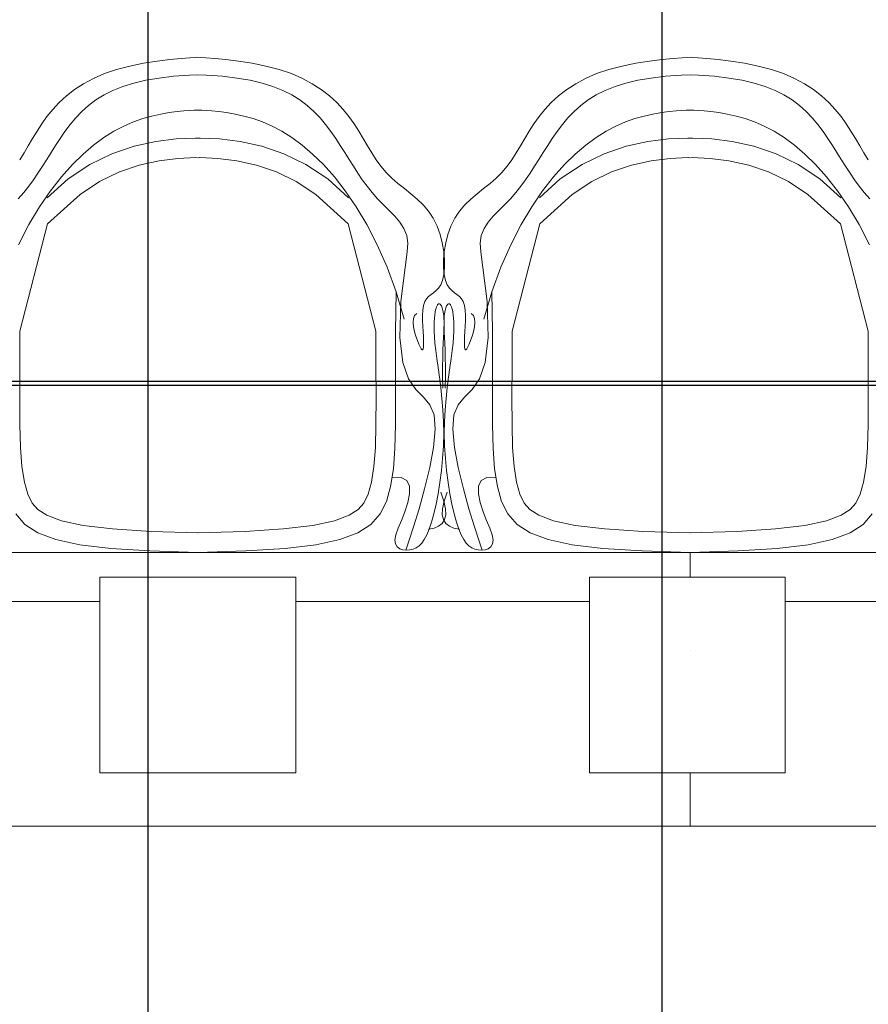
# Model space of a CAD drawing. Units: inches. Extents: x 1454 to 2136, y 626 to 1213.
# Tile 11 of 23: x 1620 to 1654, y 1101 to 1141. Entities that reach past the tile are written whole.
import ezdxf

# ---------------------------------------------------------------- set-up
doc = ezdxf.new("R2010")
doc.units = ezdxf.units.IN
doc.header["$MEASUREMENT"] = 0
for name, color, linetype, lineweight in [('A-ANNO-DIMS', 2, 'Continuous', 18), ('A-FURN-PATT', 252, 'Continuous', 13), ('conference', 41, 'Continuous', 18)]:
    doc.layers.add(name, color=color, linetype=linetype, lineweight=lineweight)
doc.styles.get("Standard").update_dxf_attribs({"font": 'arial.ttf'})
doc.dimstyles.get("Standard").update_dxf_attribs({"dimtxt": 4, "dimasz": 0.18, "dimexe": 0.18, "dimexo": 0.0625, "dimgap": 0.09, "dimtad": 0, "dimtih": 1, "dimtoh": 1, "dimdec": 0, "dimrnd": 6, "dimzin": 0, "dimdsep": 46, "dimlunit": 3, "dimtxsty": 'Standard', "dimcen": 0.09, "dimadec": 0, "dimazin": 0, "dimtfac": 1, "dimtdec": 0, "dimtofl": 0, "dimtmove": 0, "dimatfit": 3, "dimfxl": 1, "dimtolj": 1, "dimtzin": 0, "dimarcsym": 0})

# ---------------------------------------------------------------- blocks, each defined once
blk = doc.blocks.new('ОГ52_на12персон_стол2800х900')
for p, q in [((-520.6, 783.7), (-511.5, 784.5)), ((-511.5, 784.5), (-505.6, 784.9)), ((-505.6, 784.9), (-503.4, 785)), ((-501.2, 784.9), (-503.4, 785)), ((-495.2, 784.5), (-501.2, 784.9)), ((-486.2, 783.7), (-495.2, 784.5)), ((-17.8, 783.7), (-8.8, 784.5)), ((-8.8, 784.5), (-2.8, 784.9)), ((-2.8, 784.9), (-0.6, 785)), ((1.6, 784.9), (-0.6, 785)), ((7.5, 784.5), (1.6, 784.9)), ((16.6, 783.7), (7.5, 784.5)), ((-586.4, 772.5), (-572.8, 776)), ((-572.8, 776), (-558.8, 778.8)), ((-558.8, 778.8), (-544.9, 780.9)), ((-544.9, 780.9), (-531.9, 782.6)), ((-531.9, 782.6), (-520.6, 783.7)), ((-474.8, 782.6), (-486.2, 783.7)), ((-461.8, 780.9), (-474.8, 782.6)), ((-448, 778.8), (-461.8, 780.9)), ((-433.9, 776), (-448, 778.8)), ((-420.4, 772.5), (-433.9, 776)), ((-83.6, 772.5), (-70.1, 776)), ((-70.1, 776), (-56, 778.8)), ((-56, 778.8), (-42.2, 780.9)), ((-42.2, 780.9), (-29.2, 782.6)), ((-29.2, 782.6), (-17.8, 783.7)), ((27.9, 782.6), (16.6, 783.7)), ((40.9, 780.9), (27.9, 782.6)), ((54.8, 778.8), (40.9, 780.9)), ((68.8, 776), (54.8, 778.8)), ((82.4, 772.5), (68.8, 776)), ((-610.1, 763.4), (-598.8, 768.3)), ((-598.8, 768.3), (-586.4, 772.5)), ((-543.1, 763.8), (-528.3, 765.6)), ((-528.3, 765.6), (-512, 766.8)), ((-512, 766.8), (-503.4, 767.1)), ((-494.8, 766.8), (-503.4, 767.1)), ((-478.4, 765.6), (-494.8, 766.8)), ((-463.6, 763.8), (-478.4, 765.6)), ((-407.9, 768.3), (-420.4, 772.5)), ((-396.6, 763.4), (-407.9, 768.3)), ((-107.4, 763.4), (-96.1, 768.3)), ((-96.1, 768.3), (-83.6, 772.5)), ((-40.4, 763.8), (-25.6, 765.6)), ((-25.6, 765.6), (-9.3, 766.8)), ((-9.3, 766.8), (-0.6, 767.1)), ((8, 766.8), (-0.6, 767.1)), ((24.3, 765.6), (8, 766.8)), ((39.1, 763.8), (24.3, 765.6)), ((94.8, 768.3), (82.4, 772.5)), ((106.1, 763.4), (94.8, 768.3)), ((-629.5, 752), (-620.3, 758)), ((-620.3, 758), (-610.1, 763.4)), ((-590.1, 751.2), (-580, 755.2)), ((-580, 755.2), (-568.9, 758.7)), ((-568.9, 758.7), (-556.7, 761.5)), ((-556.7, 761.5), (-543.1, 763.8)), ((-450.1, 761.5), (-463.6, 763.8)), ((-437.8, 758.7), (-450.1, 761.5)), ((-426.7, 755.2), (-437.8, 758.7)), ((-416.6, 751.2), (-426.7, 755.2)), ((-386.5, 758), (-396.6, 763.4)), ((-377.3, 752), (-386.5, 758)), ((-126.7, 752), (-117.5, 758)), ((-117.5, 758), (-107.4, 763.4)), ((-87.4, 751.2), (-77.3, 755.2)), ((-77.3, 755.2), (-66.2, 758.7)), ((-66.2, 758.7), (-53.9, 761.5)), ((-53.9, 761.5), (-40.4, 763.8)), ((52.7, 761.5), (39.1, 763.8)), ((64.9, 758.7), (52.7, 761.5)), ((76, 755.2), (64.9, 758.7)), ((86.1, 751.2), (76, 755.2)), ((116.3, 758), (106.1, 763.4)), ((125.5, 752), (116.3, 758)), ((-645.1, 738.8), (-637.7, 745.6)), ((-637.7, 745.6), (-629.5, 752)), ((-607.5, 741.4), (-599.2, 746.6)), ((-599.2, 746.6), (-590.1, 751.2)), ((-407.5, 746.6), (-416.6, 751.2)), ((-399.2, 741.4), (-407.5, 746.6)), ((-369, 745.6), (-377.3, 752)), ((-361.6, 738.8), (-369, 745.6)), ((-142.4, 738.8), (-135, 745.6)), ((-135, 745.6), (-126.7, 752)), ((-104.8, 741.4), (-96.5, 746.6)), ((-96.5, 746.6), (-87.4, 751.2)), ((95.2, 746.6), (86.1, 751.2)), ((103.5, 741.4), (95.2, 746.6)), ((133.7, 745.6), (125.5, 752)), ((141.1, 738.8), (133.7, 745.6)), ((-651.7, 731.7), (-645.1, 738.8)), ((-621.9, 729.6), (-615, 735.7)), ((-615, 735.7), (-607.5, 741.4)), ((-391.7, 735.7), (-399.2, 741.4)), ((-384.9, 729.6), (-391.7, 735.7)), ((-355, 731.7), (-361.6, 738.8)), ((-149, 731.7), (-142.4, 738.8)), ((-119.1, 729.6), (-112.3, 735.7)), ((-112.3, 735.7), (-104.8, 741.4)), ((111, 735.7), (103.5, 741.4)), ((117.9, 729.6), (111, 735.7)), ((147.7, 731.7), (141.1, 738.8)), ((-662.9, 716.9), (-657.6, 724.4)), ((-657.6, 724.4), (-651.7, 731.7)), ((-628.1, 723.1), (-621.9, 729.6)), ((-559.7, 722.3), (-550.4, 724.9)), ((-550.4, 724.9), (-541.3, 727)), ((-541.3, 727), (-532.7, 728.5)), ((-532.7, 728.5), (-524.7, 729.6)), ((-524.7, 729.6), (-517.7, 730.4)), ((-517.7, 730.4), (-511.8, 730.8)), ((-511.8, 730.8), (-507.3, 731)), ((-507.3, 731), (-504.4, 731.1)), ((-504.4, 731.1), (-503.4, 731.1)), ((-502.3, 731.1), (-503.4, 731.1)), ((-499.4, 731), (-502.3, 731.1)), ((-494.9, 730.8), (-499.4, 731)), ((-489.1, 730.4), (-494.9, 730.8)), ((-482, 729.6), (-489.1, 730.4)), ((-474.1, 728.5), (-482, 729.6)), ((-465.4, 727), (-474.1, 728.5)), ((-456.3, 724.9), (-465.4, 727)), ((-447, 722.3), (-456.3, 724.9)), ((-378.6, 723.1), (-384.9, 729.6)), ((-349.1, 724.4), (-355, 731.7)), ((-343.8, 716.9), (-349.1, 724.4)), ((-160.2, 716.9), (-154.9, 724.4)), ((-154.9, 724.4), (-149, 731.7)), ((-125.4, 723.1), (-119.1, 729.6)), ((-57, 722.3), (-47.7, 724.9)), ((-47.7, 724.9), (-38.6, 727)), ((-38.6, 727), (-29.9, 728.5)), ((-29.9, 728.5), (-22, 729.6)), ((-22, 729.6), (-14.9, 730.4)), ((-14.9, 730.4), (-9.1, 730.8)), ((-9.1, 730.8), (-4.6, 731)), ((-4.6, 731), (-1.7, 731.1)), ((-1.7, 731.1), (-0.6, 731.1)), ((0.4, 731.1), (-0.6, 731.1)), ((3.3, 731), (0.4, 731.1)), ((7.8, 730.8), (3.3, 731)), ((13.7, 730.4), (7.8, 730.8)), ((20.7, 729.6), (13.7, 730.4)), ((28.7, 728.5), (20.7, 729.6)), ((37.3, 727), (28.7, 728.5)), ((46.4, 724.9), (37.3, 727)), ((55.7, 722.3), (46.4, 724.9)), ((124.1, 723.1), (117.9, 729.6)), ((153.6, 724.4), (147.7, 731.7)), ((158.9, 716.9), (153.6, 724.4)), ((-667.7, 709.4), (-662.9, 716.9)), ((-639.2, 709.3), (-633.9, 716.3)), ((-633.9, 716.3), (-628.1, 723.1)), ((-589.1, 709.4), (-579.1, 714.7)), ((-579.1, 714.7), (-569.3, 718.9)), ((-569.3, 718.9), (-559.7, 722.3)), ((-437.4, 718.9), (-447, 722.3)), ((-427.6, 714.7), (-437.4, 718.9)), ((-417.6, 709.4), (-427.6, 714.7)), ((-372.9, 716.3), (-378.6, 723.1)), ((-367.6, 709.3), (-372.9, 716.3)), ((-339, 709.4), (-343.8, 716.9)), ((-165, 709.4), (-160.2, 716.9)), ((-136.4, 709.3), (-131.1, 716.3)), ((-131.1, 716.3), (-125.4, 723.1)), ((-86.4, 709.4), (-76.4, 714.7)), ((-76.4, 714.7), (-66.6, 718.9)), ((-66.6, 718.9), (-57, 722.3)), ((65.3, 718.9), (55.7, 722.3)), ((75.1, 714.7), (65.3, 718.9)), ((85.1, 709.4), (75.1, 714.7)), ((129.8, 716.3), (124.1, 723.1)), ((135.2, 709.3), (129.8, 716.3)), ((163.7, 709.4), (158.9, 716.9)), ((-672.2, 701.9), (-667.7, 709.4)), ((-644.1, 702.2), (-639.2, 709.3)), ((-599.4, 703), (-589.1, 709.4)), ((-407.4, 703), (-417.6, 709.4)), ((-362.6, 702.2), (-367.6, 709.3)), ((-334.5, 701.9), (-339, 709.4)), ((-169.5, 701.9), (-165, 709.4)), ((-141.4, 702.2), (-136.4, 709.3)), ((-96.6, 703), (-86.4, 709.4)), ((95.4, 703), (85.1, 709.4)), ((140.1, 702.2), (135.2, 709.3)), ((168.2, 701.9), (163.7, 709.4)), ((-680.9, 687.3), (-676.6, 694.5)), ((-676.6, 694.5), (-672.2, 701.9)), ((-653.4, 687.9), (-648.8, 695)), ((-648.8, 695), (-644.1, 702.2)), ((-620.6, 686.1), (-609.9, 695.3)), ((-609.9, 695.3), (-599.4, 703)), ((-591.2, 686.5), (-568.6, 694.2)), ((-568.6, 694.2), (-546.5, 699)), ((-546.5, 699), (-525.4, 701.6)), ((-525.4, 701.6), (-505.7, 702.5)), ((-505.7, 702.5), (-503.4, 702.4)), ((-501, 702.5), (-503.4, 702.4)), ((-481.3, 701.6), (-501, 702.5)), ((-460.2, 699), (-481.3, 701.6)), ((-438.1, 694.2), (-460.2, 699)), ((-415.6, 686.5), (-438.1, 694.2)), ((-396.9, 695.3), (-407.4, 703)), ((-386.2, 686.1), (-396.9, 695.3)), ((-357.9, 695), (-362.6, 702.2)), ((-353.4, 687.9), (-357.9, 695)), ((-330.2, 694.5), (-334.5, 701.9)), ((-325.8, 687.3), (-330.2, 694.5)), ((-178.2, 687.3), (-173.9, 694.5)), ((-173.9, 694.5), (-169.5, 701.9)), ((-150.6, 687.9), (-146.1, 695)), ((-146.1, 695), (-141.4, 702.2)), ((-117.9, 686.1), (-107.1, 695.3)), ((-107.1, 695.3), (-96.6, 703)), ((-88.4, 686.5), (-65.9, 694.2)), ((-65.9, 694.2), (-43.8, 699)), ((-43.8, 699), (-22.7, 701.6)), ((-22.7, 701.6), (-3, 702.5)), ((-3, 702.5), (-0.6, 702.4)), ((1.7, 702.5), (-0.6, 702.4)), ((21.4, 701.6), (1.7, 702.5)), ((42.5, 699), (21.4, 701.6)), ((64.6, 694.2), (42.5, 699)), ((87.2, 686.5), (64.6, 694.2)), ((105.9, 695.3), (95.4, 703)), ((116.6, 686.1), (105.9, 695.3)), ((144.8, 695), (140.1, 702.2)), ((149.4, 687.9), (144.8, 695)), ((172.6, 694.5), (168.2, 701.9)), ((176.9, 687.3), (172.6, 694.5)), ((-685.4, 680.3), (-680.9, 687.3)), ((-657.8, 680.7), (-653.4, 687.9)), ((-631.5, 675.4), (-620.6, 686.1)), ((-613.8, 675.6), (-591.2, 686.5)), ((-393, 675.6), (-415.6, 686.5)), ((-375.2, 675.4), (-386.2, 686.1)), ((-348.9, 680.7), (-353.4, 687.9)), ((-321.3, 680.3), (-325.8, 687.3)), ((-182.7, 680.3), (-178.2, 687.3)), ((-155.1, 680.7), (-150.6, 687.9)), ((-128.8, 675.4), (-117.9, 686.1)), ((-111, 675.6), (-88.4, 686.5)), ((109.8, 675.6), (87.2, 686.5)), ((127.5, 675.4), (116.6, 686.1)), ((153.8, 680.7), (149.4, 687.9)), ((181.4, 680.3), (176.9, 687.3)), ((-666.7, 666.7), (-662.2, 673.7)), ((-662.2, 673.7), (-657.8, 680.7)), ((-642.7, 663), (-631.5, 675.4)), ((-636, 660.8), (-613.8, 675.6)), ((-583.6, 668), (-563.2, 674.9)), ((-563.2, 674.9), (-543.1, 679.3)), ((-543.1, 679.3), (-523.8, 681.7)), ((-523.8, 681.7), (-505.5, 682.5)), ((-505.5, 682.5), (-503.8, 682.4)), ((-501.3, 682.5), (-503, 682.4)), ((-483, 681.7), (-501.3, 682.5)), ((-463.6, 679.3), (-483, 681.7)), ((-443.5, 674.9), (-463.6, 679.3)), ((-423.2, 668), (-443.5, 674.9)), ((-370.7, 660.8), (-393, 675.6)), ((-364, 663), (-375.2, 675.4)), ((-344.5, 673.7), (-348.9, 680.7)), ((-340.1, 666.7), (-344.5, 673.7)), ((-316.5, 673.7), (-321.3, 680.3)), ((-311.2, 667.5), (-316.5, 673.7)), ((-192.8, 667.5), (-187.5, 673.7)), ((-187.5, 673.7), (-182.7, 680.3)), ((-163.9, 666.7), (-159.5, 673.7)), ((-159.5, 673.7), (-155.1, 680.7)), ((-140, 663), (-128.8, 675.4)), ((-133.3, 660.8), (-111, 675.6)), ((-80.8, 668), (-60.5, 674.9)), ((-60.5, 674.9), (-40.4, 679.3)), ((-40.4, 679.3), (-21, 681.7)), ((-21, 681.7), (-2.7, 682.5)), ((-2.7, 682.5), (-1, 682.4)), ((1.5, 682.5), (-0.2, 682.4)), ((19.7, 681.7), (1.5, 682.5)), ((39.1, 679.3), (19.7, 681.7)), ((59.2, 674.9), (39.1, 679.3)), ((79.6, 668), (59.2, 674.9)), ((132, 660.8), (109.8, 675.6)), ((138.7, 663), (127.5, 675.4)), ((158.2, 673.7), (153.8, 680.7)), ((162.7, 666.7), (158.2, 673.7)), ((-671.3, 659.9), (-666.7, 666.7)), ((-603.8, 658.2), (-583.6, 668)), ((-402.9, 658.2), (-423.2, 668)), ((-335.5, 659.9), (-340.1, 666.7)), ((-305.3, 661.7), (-311.2, 667.5)), ((-198.7, 661.7), (-192.8, 667.5)), ((-168.6, 659.9), (-163.9, 666.7)), ((-101.1, 658.2), (-80.8, 668)), ((99.8, 658.2), (79.6, 668)), ((167.3, 659.9), (162.7, 666.7)), ((-676.1, 653.3), (-671.3, 659.9)), ((-657.3, 641.6), (-636, 660.8)), ((-654, 648.7), (-642.7, 663)), ((-623.7, 644.9), (-603.8, 658.2)), ((-383, 644.9), (-402.9, 658.2)), ((-349.4, 641.6), (-370.7, 660.8)), ((-352.8, 648.7), (-364, 663)), ((-330.6, 653.3), (-335.5, 659.9)), ((-299, 656.2), (-305.3, 661.7)), ((-292.5, 650.9), (-299, 656.2)), ((-211.5, 650.9), (-205, 656.2)), ((-205, 656.2), (-198.7, 661.7)), ((-173.4, 653.3), (-168.6, 659.9)), ((-154.6, 641.6), (-133.3, 660.8)), ((-151.3, 648.7), (-140, 663)), ((-121, 644.9), (-101.1, 658.2)), ((119.7, 644.9), (99.8, 658.2)), ((153.3, 641.6), (132, 660.8)), ((150, 648.7), (138.7, 663)), ((172.1, 653.3), (167.3, 659.9)), ((-686.8, 640.6), (-681.3, 646.8)), ((-681.3, 646.8), (-676.1, 653.3)), ((-665.2, 632.4), (-654, 648.7)), ((-657, 615), (-623.7, 644.9)), ((-349.8, 615), (-383, 644.9)), ((-341.6, 632.4), (-352.8, 648.7)), ((-325.5, 646.8), (-330.6, 653.3)), ((-320, 640.6), (-325.5, 646.8)), ((-285.9, 645.6), (-292.5, 650.9)), ((-279.5, 640.1), (-285.9, 645.6)), ((-224.5, 640.1), (-218.1, 645.6)), ((-218.1, 645.6), (-211.5, 650.9)), ((-184, 640.6), (-178.5, 646.8)), ((-178.5, 646.8), (-173.4, 653.3)), ((-162.4, 632.4), (-151.3, 648.7)), ((-154.2, 615), (-121, 644.9)), ((153, 615), (119.7, 644.9)), ((161.2, 632.4), (150, 648.7)), ((177.3, 646.8), (172.1, 653.3)), ((182.8, 640.6), (177.3, 646.8)), ((-314.1, 634.6), (-320, 640.6)), ((-308, 628.7), (-314.1, 634.6)), ((-273.4, 634.2), (-279.5, 640.1)), ((-267.8, 627.7), (-273.4, 634.2)), ((-236.2, 627.7), (-230.6, 634.2)), ((-230.6, 634.2), (-224.5, 640.1)), ((-196, 628.7), (-190, 634.6)), ((-190, 634.6), (-184, 640.6)), ((-676.1, 614.1), (-665.2, 632.4)), ((-330.7, 614.1), (-341.6, 632.4)), ((-302.3, 622.8), (-308, 628.7)), ((-263, 620.6), (-267.8, 627.7)), ((-241, 620.6), (-236.2, 627.7)), ((-201.7, 622.8), (-196, 628.7)), ((-173.3, 614.1), (-162.4, 632.4)), ((172.1, 614.1), (161.2, 632.4)), ((-686.6, 593.6), (-676.1, 614.1)), ((-657, 615), (-685.3, 505.2)), ((-349.8, 615), (-321.5, 505.2)), ((-320.1, 593.6), (-330.7, 614.1)), ((-297.1, 616.6), (-302.3, 622.8)), ((-292.9, 610.1), (-297.1, 616.6)), ((-259.1, 612.7), (-263, 620.6)), ((-244.9, 612.7), (-241, 620.6)), ((-211.1, 610.1), (-206.9, 616.6)), ((-206.9, 616.6), (-201.7, 622.8)), ((-183.9, 593.6), (-173.3, 614.1)), ((-154.2, 615), (-182.5, 505.2)), ((153, 615), (181.3, 505.2)), ((182.6, 593.6), (172.1, 614.1)), ((-290, 603), (-292.9, 610.1)), ((-256, 604.2), (-259.1, 612.7)), ((-253.8, 595.4), (-256, 604.2)), ((-250.2, 595.4), (-248, 604.2)), ((-248, 604.2), (-244.9, 612.7)), ((-214, 603), (-211.1, 610.1)), ((-310.2, 570.7), (-320.1, 593.6)), ((-288.8, 595.2), (-290, 603)), ((-289.6, 586.5), (-288.8, 595.2)), ((-252.3, 586.6), (-253.8, 595.4)), ((-251.7, 586.6), (-250.2, 595.4)), ((-215.2, 595.2), (-214, 603)), ((-214.4, 586.5), (-215.2, 595.2)), ((-193.8, 570.7), (-183.9, 593.6)), ((-289.6, 586.5), (-296, 535.5)), ((-252.4, 578.1), (-251.7, 586.6)), ((-251.6, 578.1), (-252.3, 586.6)), ((-214.4, 586.5), (-208, 535.5)), ((-252.4, 570.2), (-252.4, 578.1)), ((-251.6, 570.2), (-251.6, 578.1)), ((-301, 545.4), (-310.2, 570.7)), ((-253.5, 557.2), (-252.3, 563.1)), ((-251.7, 563.1), (-252.4, 570.2)), ((-252.3, 563.1), (-251.6, 570.2)), ((-250.5, 557.2), (-251.7, 563.1)), ((-203, 545.4), (-193.8, 570.7)), ((-255.3, 552.7), (-253.5, 557.2)), ((-248.7, 552.7), (-250.5, 557.2)), ((-301, 545.4), (-301.5, 505.1)), ((-292.7, 517.6), (-301, 545.4)), ((-265.2, 542.8), (-262.6, 544.6)), ((-262.6, 544.6), (-260, 546.7)), ((-260, 546.7), (-257.5, 549.3)), ((-257.5, 549.3), (-255.3, 552.7)), ((-246.5, 549.3), (-248.7, 552.7)), ((-244, 546.7), (-246.5, 549.3)), ((-241.4, 544.6), (-244, 546.7)), ((-238.8, 542.8), (-241.4, 544.6)), ((-211.3, 517.6), (-203, 545.4)), ((-203, 545.4), (-202.5, 505.1)), ((-296, 535.5), (-297, 498.8)), ((-272.8, 531.5), (-271.6, 535.5)), ((-271.6, 535.5), (-269.8, 538.5)), ((-269.8, 538.5), (-267.7, 540.8)), ((-267.7, 540.8), (-265.2, 542.8)), ((-258.6, 532.3), (-258.1, 532.9)), ((-258.1, 532.9), (-257.6, 533.2)), ((-257.6, 533.2), (-257, 533.3)), ((-257, 533.3), (-256.5, 533.2)), ((-256.5, 533.2), (-256, 533)), ((-256, 533), (-255.6, 532.5)), ((-248, 533), (-248.4, 532.5)), ((-247.5, 533.2), (-248, 533)), ((-247, 533.3), (-247.5, 533.2)), ((-246.4, 533.2), (-247, 533.3)), ((-245.9, 532.9), (-246.4, 533.2)), ((-245.4, 532.3), (-245.9, 532.9)), ((-236.3, 540.8), (-238.8, 542.8)), ((-234.2, 538.5), (-236.3, 540.8)), ((-232.4, 535.5), (-234.2, 538.5)), ((-231.2, 531.5), (-232.4, 535.5)), ((-208, 535.5), (-207, 498.8)), ((-279.9, 523.4), (-282.1, 521.4)), ((-273.8, 521.5), (-273.5, 526.8)), ((-273.5, 526.8), (-272.8, 531.5)), ((-261.4, 521.9), (-261, 524.7)), ((-261, 524.7), (-260.6, 527)), ((-260.6, 527), (-260.1, 528.8)), ((-260.1, 528.8), (-259.6, 530.3)), ((-259.6, 530.3), (-259.1, 531.5)), ((-259.1, 531.5), (-258.6, 532.3)), ((-255.6, 532.5), (-255.1, 531.9)), ((-255.1, 531.9), (-254.7, 531.1)), ((-254.7, 531.1), (-254.2, 530.2)), ((-254.2, 530.2), (-253.8, 529.1)), ((-253.8, 529.1), (-253.5, 527.9)), ((-253.5, 527.9), (-253.1, 526.5)), ((-253.1, 526.5), (-252.8, 524.9)), ((-252.8, 524.9), (-252.5, 523.1)), ((-252.5, 523.1), (-252.3, 521)), ((-251.5, 523.1), (-251.7, 521)), ((-251.2, 524.9), (-251.5, 523.1)), ((-250.9, 526.5), (-251.2, 524.9)), ((-250.6, 527.9), (-250.9, 526.5)), ((-250.2, 529.1), (-250.6, 527.9)), ((-249.8, 530.2), (-250.2, 529.1)), ((-249.3, 531.1), (-249.8, 530.2)), ((-248.9, 531.9), (-249.3, 531.1)), ((-248.4, 532.5), (-248.9, 531.9)), ((-244.9, 531.5), (-245.4, 532.3)), ((-244.4, 530.3), (-244.9, 531.5)), ((-243.9, 528.8), (-244.4, 530.3)), ((-243.4, 527), (-243.9, 528.8)), ((-243, 524.7), (-243.4, 527)), ((-242.6, 521.9), (-243, 524.7)), ((-230.5, 526.8), (-231.2, 531.5)), ((-230.2, 521.5), (-230.5, 526.8)), ((-224.1, 523.4), (-221.9, 521.4)), ((-283.2, 518.2), (-283.5, 514.2)), ((-283.5, 514.2), (-283, 509.6)), ((-282.1, 521.4), (-283.2, 518.2)), ((-273.8, 516), (-273.8, 521.5)), ((-273.6, 510.3), (-273.8, 516)), ((-262, 510.5), (-261.9, 514.9)), ((-261.9, 514.9), (-261.7, 518.7)), ((-261.7, 518.7), (-261.4, 521.9)), ((-252.3, 521), (-252.1, 518.5)), ((-252.1, 518.5), (-252, 515.7)), ((-251.9, 518.5), (-252, 515.7)), ((-252, 515.7), (-252, 512.3)), ((-252, 515.7), (-252, 512.3)), ((-251.7, 521), (-251.9, 518.5)), ((-242.3, 518.7), (-242.6, 521.9)), ((-242.1, 514.9), (-242.3, 518.7)), ((-242, 510.5), (-242.1, 514.9)), ((-230.4, 510.3), (-230.2, 516)), ((-230.2, 516), (-230.2, 521.5)), ((-221.9, 521.4), (-220.8, 518.2)), ((-220.5, 514.2), (-221, 509.6)), ((-220.8, 518.2), (-220.5, 514.2)), ((-685.3, 505.2), (-685.3, 469.2)), ((-321.5, 505.2), (-321.5, 469.2)), ((-301.5, 505.1), (-301.5, 469.2)), ((-283, 509.6), (-282, 504.8)), ((-282, 504.8), (-280.7, 500.1)), ((-273.4, 504.9), (-273.6, 510.3)), ((-273.1, 499.8), (-273.4, 504.9)), ((-262, 505.4), (-262, 510.5)), ((-261.7, 499.6), (-262, 505.4)), ((-252.3, 504), (-252.5, 498.9)), ((-252.1, 508.5), (-252.3, 504)), ((-252, 512.3), (-252.1, 508.5)), ((-252, 512.3), (-251.9, 508.5)), ((-251.9, 508.5), (-251.7, 504)), ((-251.7, 504), (-251.5, 498.9)), ((-242.3, 499.6), (-242, 505.4)), ((-242, 505.4), (-242, 510.5)), ((-230.9, 499.8), (-230.6, 504.9)), ((-230.6, 504.9), (-230.4, 510.3)), ((-222, 504.8), (-223.3, 500.1)), ((-221, 509.6), (-222, 504.8)), ((-202.5, 505.1), (-202.5, 469.2)), ((-182.5, 505.2), (-182.5, 469.2)), ((181.3, 505.2), (181.3, 469.2)), ((-297, 498.8), (-294, 473.4)), ((-280.7, 500.1), (-279.2, 495.7)), ((-279.2, 495.7), (-277.7, 492)), ((-272.9, 495.4), (-273.1, 499.8)), ((-272.8, 491.8), (-272.9, 495.4)), ((-261.2, 493.1), (-261.7, 499.6)), ((-260.4, 485.6), (-261.2, 493.1)), ((-252.8, 493), (-253.1, 486.1)), ((-252.5, 498.9), (-252.8, 493)), ((-251.5, 498.9), (-251.2, 493)), ((-251.2, 493), (-250.9, 486.1)), ((-243.6, 485.6), (-242.8, 493.1)), ((-242.8, 493.1), (-242.3, 499.6)), ((-231.2, 491.8), (-231.1, 495.4)), ((-231.1, 495.4), (-230.9, 499.8)), ((-224.8, 495.7), (-226.3, 492)), ((-223.3, 500.1), (-224.8, 495.7)), ((-207, 498.8), (-210.1, 473.4)), ((-277.7, 492), (-276.4, 489.2)), ((-276.4, 489.2), (-275.3, 487.3)), ((-275.3, 487.3), (-274.4, 486.4)), ((-274.4, 486.4), (-273.8, 486.4)), ((-273.8, 486.4), (-273.3, 487.3)), ((-273.3, 487.3), (-272.9, 489.1)), ((-272.9, 489.1), (-272.8, 491.8)), ((-259.3, 477.3), (-260.4, 485.6)), ((-253.1, 486.1), (-253.3, 478.2)), ((-250.9, 486.1), (-250.7, 478.2)), ((-244.7, 477.3), (-243.6, 485.6)), ((-231.1, 489.1), (-231.2, 491.8)), ((-230.7, 487.3), (-231.1, 489.1)), ((-230.3, 486.4), (-230.7, 487.3)), ((-229.6, 486.4), (-230.3, 486.4)), ((-228.7, 487.3), (-229.6, 486.4)), ((-227.6, 489.2), (-228.7, 487.3)), ((-226.3, 492), (-227.6, 489.2)), ((-294, 473.4), (-288.1, 456.6)), ((-258, 468.2), (-259.3, 477.3)), ((-253.3, 478.2), (-253.4, 469.2)), ((-250.7, 478.2), (-250.6, 469.2)), ((-246, 468.2), (-244.7, 477.3)), ((-210.1, 473.4), (-215.9, 456.6)), ((-685.3, 469.2), (-685.4, 437.6)), ((-321.5, 469.2), (-321.4, 437.6)), ((-301.5, 469.2), (-301.4, 437.5)), ((-256.7, 458.3), (-258, 468.2)), ((-253.4, 469.2), (-253.5, 458.8)), ((-250.6, 469.2), (-250.5, 458.8)), ((-247.3, 458.3), (-246, 468.2)), ((-202.5, 469.2), (-202.6, 437.5)), ((-182.5, 469.2), (-182.6, 437.6)), ((181.3, 469.2), (181.4, 437.6)), ((-288.1, 456.6), (-280.7, 445.7)), ((-255.4, 447.8), (-256.7, 458.3)), ((-253.5, 458.8), (-253.3, 447.1)), ((-250.5, 458.8), (-250.7, 447.1)), ((-248.7, 447.8), (-247.3, 458.3)), ((-215.9, 456.6), (-223.3, 445.7)), ((-280.7, 445.7), (-273.1, 437.8)), ((-254.1, 436.7), (-255.4, 447.8)), ((-249.9, 436.7), (-248.7, 447.8)), ((-223.3, 445.7), (-230.9, 437.8)), ((-685.4, 437.6), (-685.3, 410.1)), ((-321.4, 437.6), (-321.5, 410.1)), ((-301.4, 437.5), (-301.5, 409.8)), ((-273.1, 437.8), (-266.5, 430.2)), ((-253.1, 425.1), (-254.1, 436.7)), ((-250.9, 425.1), (-249.9, 436.7)), ((-230.9, 437.8), (-237.5, 430.2)), ((-202.6, 437.5), (-202.5, 409.8)), ((-182.6, 437.6), (-182.5, 410.1)), ((181.4, 437.6), (181.2, 410.1)), ((-266.5, 430.2), (-262.2, 420)), ((-252.5, 413.1), (-253.1, 425.1)), ((-251.5, 413.1), (-250.9, 425.1)), ((-237.5, 430.2), (-241.8, 420)), ((-262.2, 420), (-261.1, 405.3)), ((-252.3, 400.7), (-252.5, 413.1)), ((-251.7, 400.7), (-251.5, 413.1)), ((-241.8, 420), (-242.9, 405.3)), ((-685.3, 410.1), (-684.6, 386.6)), ((-321.5, 410.1), (-322.1, 386.6)), ((-301.5, 409.8), (-302.2, 385.6)), ((-261.1, 405.3), (-262.8, 386.7)), ((-242.9, 405.3), (-241.2, 386.7)), ((-202.5, 409.8), (-201.8, 385.6)), ((-182.5, 410.1), (-181.9, 386.6)), ((181.2, 410.1), (180.6, 386.6)), ((-252.6, 388.2), (-252.3, 400.7)), ((-251.4, 388.2), (-251.7, 400.7)), ((-684.6, 386.6), (-683.1, 367)), ((-322.1, 386.6), (-323.6, 367)), ((-302.2, 385.6), (-303.7, 364.7)), ((-262.8, 386.7), (-266.6, 366)), ((-253.4, 375.5), (-252.6, 388.2)), ((-250.6, 375.5), (-251.4, 388.2)), ((-241.2, 386.7), (-237.4, 366)), ((-201.8, 385.6), (-200.3, 364.7)), ((-181.9, 386.6), (-180.4, 367)), ((180.6, 386.6), (179.1, 367)), ((-254.6, 363), (-253.4, 375.5)), ((-249.4, 363), (-250.6, 375.5)), ((-683.1, 367), (-680.6, 351.1)), ((-323.6, 367), (-326.1, 351.1)), ((-303.7, 364.7), (-306.5, 346.8)), ((-266.6, 366), (-271.8, 344.5)), ((-256.2, 350.9), (-254.6, 363)), ((-247.8, 350.9), (-249.4, 363)), ((-237.4, 366), (-232.2, 344.5)), ((-200.3, 364.7), (-197.5, 346.8)), ((-180.4, 367), (-177.9, 351.1)), ((179.1, 367), (176.6, 351.1)), ((-295.6, 356.1), (-305.1, 355.7)), ((-289.9, 353), (-295.6, 356.1)), ((-287.3, 347.1), (-289.9, 353)), ((-216.7, 347.1), (-214.1, 353)), ((-214.1, 353), (-208.4, 356.1)), ((-208.4, 356.1), (-198.9, 355.7)), ((-680.6, 351.1), (-677.1, 338.8)), ((-326.1, 351.1), (-329.6, 338.8)), ((-306.5, 346.8), (-310.9, 331.5)), ((-287.3, 339.3), (-287.3, 347.1)), ((-271.8, 344.5), (-277.5, 323.8)), ((-258, 339.4), (-256.2, 350.9)), ((-246, 339.4), (-247.8, 350.9)), ((-232.2, 344.5), (-226.5, 323.8)), ((-216.7, 339.3), (-216.7, 347.1)), ((-197.5, 346.8), (-193.1, 331.5)), ((-177.9, 351.1), (-174.4, 338.8)), ((176.6, 351.1), (173.1, 338.8)), ((-677.1, 338.8), (-672.7, 329.9)), ((-329.6, 338.8), (-334, 329.9)), ((-289.1, 330.3), (-287.3, 339.3)), ((-260.1, 328.7), (-258, 339.4)), ((-255.4, 341), (-252.1, 331.8)), ((-251.9, 331.8), (-253.6, 324.1)), ((-252.1, 331.8), (-250.4, 324.1)), ((-248.6, 341), (-251.9, 331.8)), ((-243.9, 328.7), (-246, 339.4)), ((-214.9, 330.3), (-216.7, 339.3)), ((-174.4, 338.8), (-170, 329.9)), ((173.1, 338.8), (168.7, 329.9)), ((-672.7, 329.9), (-666.9, 323.3)), ((-666.9, 323.3), (-657.8, 317.4)), ((-339.8, 323.3), (-349, 317.4)), ((-334, 329.9), (-339.8, 323.3)), ((-310.9, 331.5), (-317.3, 318.7)), ((-292, 321), (-289.1, 330.3)), ((-277.5, 323.8), (-283.1, 305.4)), ((-262.3, 318.9), (-260.1, 328.7)), ((-253.6, 324.1), (-253.8, 317.8)), ((-250.4, 324.1), (-250.2, 317.8)), ((-241.7, 318.9), (-243.9, 328.7)), ((-226.5, 323.8), (-220.9, 305.4)), ((-212, 321), (-214.9, 330.3)), ((-193.1, 331.5), (-186.7, 318.7)), ((-170, 329.9), (-164.2, 323.3)), ((-164.2, 323.3), (-155.1, 317.4)), ((162.9, 323.3), (153.8, 317.4)), ((168.7, 329.9), (162.9, 323.3)), ((-689.5, 318.7), (-680.2, 308)), ((-657.8, 317.4), (-642.8, 311.8)), ((-642.8, 311.8), (-620.7, 307)), ((-363.9, 311.8), (-386.1, 307)), ((-349, 317.4), (-363.9, 311.8)), ((-317.3, 318.7), (-326.6, 308)), ((-298.9, 304.2), (-295.5, 312)), ((-295.5, 312), (-292, 321)), ((-264.7, 310.4), (-262.3, 318.9)), ((-251.5, 312.9), (-254, 309)), ((-253.8, 317.8), (-252.5, 312.9)), ((-252.5, 312.9), (-250, 309)), ((-250.2, 317.8), (-251.5, 312.9)), ((-239.3, 310.4), (-241.7, 318.9)), ((-208.5, 312), (-212, 321)), ((-205.1, 304.2), (-208.5, 312)), ((-186.7, 318.7), (-177.4, 308)), ((-155.1, 317.4), (-140.1, 311.8)), ((-140.1, 311.8), (-117.9, 307)), ((138.8, 311.8), (116.7, 307)), ((153.8, 317.4), (138.8, 311.8)), ((185.5, 318.7), (176.2, 308)), ((-680.2, 308), (-666.8, 299.4)), ((-620.7, 307), (-590.5, 303.4)), ((-590.5, 303.4), (-551.5, 300.9)), ((-416.3, 303.4), (-455.2, 300.9)), ((-386.1, 307), (-416.3, 303.4)), ((-326.6, 308), (-339.9, 299.4)), ((-298.9, 304.2), (-301.3, 297.4)), ((-283.1, 305.4), (-287.8, 291)), ((-269.5, 297.3), (-267.1, 303.2)), ((-262.2, 304.3), (-267.7, 303.1)), ((-267.1, 303.2), (-264.7, 310.4)), ((-257.6, 306.2), (-262.2, 304.3)), ((-254, 309), (-257.6, 306.2)), ((-250, 309), (-246.4, 306.2)), ((-246.4, 306.2), (-241.8, 304.3)), ((-241.8, 304.3), (-236.3, 303.1)), ((-236.9, 303.2), (-239.3, 310.4)), ((-234.5, 297.3), (-236.9, 303.2)), ((-220.9, 305.4), (-216.2, 291)), ((-205.1, 304.2), (-202.7, 297.4)), ((-177.4, 308), (-164.1, 299.4)), ((-117.9, 307), (-87.8, 303.4)), ((-87.8, 303.4), (-48.8, 300.9)), ((86.5, 303.4), (47.5, 300.9)), ((116.7, 307), (86.5, 303.4)), ((176.2, 308), (162.8, 299.4)), ((-666.8, 299.4), (-648.5, 292.5)), ((-648.5, 292.5), (-624, 287.3)), ((-551.5, 300.9), (-502.7, 299.3)), ((-455.2, 300.9), (-504, 299.3)), ((-358.3, 292.5), (-382.8, 287.3)), ((-339.9, 299.4), (-358.3, 292.5)), ((-301.3, 297.4), (-302.1, 292.1)), ((-302.1, 292.1), (-301.5, 288.1)), ((-274.7, 288.8), (-272.1, 292.5)), ((-272.1, 292.5), (-269.5, 297.3)), ((-231.9, 292.5), (-234.5, 297.3)), ((-229.3, 288.8), (-231.9, 292.5)), ((-202.7, 297.4), (-201.9, 292.1)), ((-201.9, 292.1), (-202.5, 288.1)), ((-164.1, 299.4), (-145.7, 292.5)), ((-145.7, 292.5), (-121.2, 287.3)), ((-48.8, 300.9), (0, 299.3)), ((47.5, 300.9), (-1.3, 299.3)), ((144.5, 292.5), (120, 287.3)), ((162.8, 299.4), (144.5, 292.5)), ((-624, 287.3), (-592.3, 283.5)), ((-592.3, 283.5), (-552.5, 280.9)), ((-414.4, 283.5), (-454.3, 280.9)), ((-382.8, 287.3), (-414.4, 283.5)), ((-301.5, 288.1), (-299.7, 285.1)), ((-299.7, 285.1), (-297.1, 283.2)), ((-297.1, 283.2), (-293.9, 282.2)), ((-293.9, 282.2), (-290.4, 281.8)), ((-287.8, 291), (-290.9, 281.9)), ((-290.4, 281.8), (-286.9, 282.1)), ((-286.9, 282.1), (-283.6, 282.8)), ((-283.6, 282.8), (-280.4, 284.1)), ((-280.4, 284.1), (-277.5, 286.1)), ((-277.5, 286.1), (-274.7, 288.8)), ((-226.5, 286.1), (-229.3, 288.8)), ((-223.6, 284.1), (-226.5, 286.1)), ((-220.4, 282.8), (-223.6, 284.1)), ((-217.1, 282.1), (-220.4, 282.8)), ((-213.6, 281.8), (-217.1, 282.1)), ((-216.2, 291), (-213.1, 281.9)), ((-210.1, 282.2), (-213.6, 281.8)), ((-206.9, 283.2), (-210.1, 282.2)), ((-204.3, 285.1), (-206.9, 283.2)), ((-202.5, 288.1), (-204.3, 285.1)), ((-121.2, 287.3), (-89.6, 283.5)), ((-89.6, 283.5), (-49.7, 280.9)), ((88.3, 283.5), (48.5, 280.9)), ((120, 287.3), (88.3, 283.5)), ((-1300, 279.3), (1300, 279.3)), ((-552.5, 280.9), (-503.4, 279.3)), ((-454.3, 280.9), (-503.4, 279.3)), ((-49.7, 280.9), (-0.6, 279.3)), ((48.5, 280.9), (-0.6, 279.3)), ((-0.6, 279.3), (-0.6, 254.3)), ((-603.4, 254.3), (-603.4, 54.3)), ((-403.4, 254.3), (-603.4, 254.3)), ((-403.4, 54.3), (-403.4, 254.3)), ((-103.4, 254.3), (-103.4, 54.3)), ((96.6, 254.3), (-103.4, 254.3)), ((96.6, 54.3), (96.6, 254.3)), ((-603.4, 229.3), (-903.4, 229.3)), ((-103.4, 229.3), (-403.4, 229.3)), ((403.4, 229.3), (96.6, 229.3)), ((0, 179.3), (0, 179.3)), ((0, 179.3), (0, 179.3)), ((-603.4, 54.3), (-403.4, 54.3)), ((-103.4, 54.3), (96.6, 54.3)), ((-0.6, 54.3), (-0.6, 0)), ((1220.7, 0), (-1220.7, 0))]:
    blk.add_line(p, q)
blk = doc.blocks.new('*D23')
at = {"layer": 'A-ANNO-DIMS', "color": 0, "lineweight": -2, "transparency": 16777216}
for p, q in [((1571.674, 1139.532), (1571.674, 1162.157)), ((1721.725, 1139.532), (1721.725, 1162.157)), ((1571.854, 1161.977), (1615.675, 1161.977)), ((1721.545, 1161.977), (1677.724, 1161.977))]:
    blk.add_line(p, q, dxfattribs=at)
at = {"layer": 'A-ANNO-DIMS', "color": 0, "transparency": 16777216}
for points in [[(1571.854, 1162.007), (1571.854, 1161.947), (1571.674, 1161.977)], [(1721.545, 1162.007), (1721.545, 1161.947), (1721.725, 1161.977)]]:
    blk.add_solid(points, dxfattribs=at)
at = {"layer": 'Defpoints', "color": 0, "transparency": 16777216}
for p in [(1721.725, 1161.977), (1571.674, 1139.469), (1721.725, 1139.469)]:
    blk.add_point(p, dxfattribs=at)
at = {"layer": 'A-ANNO-DIMS', "color": 0, "transparency": 16777216, "insert": (1646.7, 1161.977), "char_height": 4, "attachment_point": 5}
blk.add_mtext('\\A1;CONFERENCE SET 150', dxfattribs=at)
blk = doc.blocks.new('*D33')
at = {"layer": 'A-ANNO-DIMS', "color": 0, "lineweight": -2, "transparency": 16777216}
for p, q in [((2032.494, 1126.282), (1462.374, 1126.282)), ((1462.554, 1126.102), (1462.554, 1056.381)), ((1462.554, 982.462), (1462.554, 1052.184)), ((2032.494, 982.282), (1462.374, 982.282))]:
    blk.add_line(p, q, dxfattribs=at)
at = {"layer": 'A-ANNO-DIMS', "color": 0, "transparency": 16777216}
for points in [[(1462.524, 1126.102), (1462.584, 1126.102), (1462.554, 1126.282)], [(1462.524, 982.462), (1462.584, 982.462), (1462.554, 982.282)]]:
    blk.add_solid(points, dxfattribs=at)
at = {"layer": 'Defpoints', "color": 0, "transparency": 16777216}
for p in [(1462.554, 1126.282), (2032.556, 1126.282), (2032.556, 982.282)]:
    blk.add_point(p, dxfattribs=at)
at = {"layer": 'A-ANNO-DIMS', "color": 0, "transparency": 16777216, "insert": (1462.554, 1054.282), "char_height": 4, "attachment_point": 5}
blk.add_mtext('\\A1;144', dxfattribs=at)
blk = doc.blocks.new('*D40')
at = {"layer": 'A-ANNO-DIMS', "color": 0, "lineweight": -2, "transparency": 16777216}
for p, q in [((1501.556, 877.345), (1501.556, 1210.464)), ((1501.736, 1210.284), (1569.244, 1210.284)), ((1645.376, 1210.284), (1577.869, 1210.284)), ((1645.556, 877.345), (1645.556, 1210.464))]:
    blk.add_line(p, q, dxfattribs=at)
at = {"layer": 'A-ANNO-DIMS', "color": 0, "transparency": 16777216}
for points in [[(1501.736, 1210.314), (1501.736, 1210.254), (1501.556, 1210.284)], [(1645.376, 1210.314), (1645.376, 1210.254), (1645.556, 1210.284)]]:
    blk.add_solid(points, dxfattribs=at)
at = {"layer": 'Defpoints', "color": 0, "transparency": 16777216}
for p in [(1645.556, 1210.284), (1501.556, 877.282), (1645.556, 877.282)]:
    blk.add_point(p, dxfattribs=at)
at = {"layer": 'A-ANNO-DIMS', "color": 0, "transparency": 16777216, "insert": (1573.556, 1210.284), "char_height": 4, "attachment_point": 5}
blk.add_mtext('\\A1;144', dxfattribs=at)
blk = doc.blocks.new('*D54')
at = {"layer": 'A-ANNO-DIMS', "color": 0, "lineweight": -2, "transparency": 16777216}
for p, q in [((1879.494, 1126.282), (1462.374, 1126.282)), ((1462.554, 1126.102), (1462.554, 1078.915)), ((1462.554, 1027.462), (1462.554, 1074.65)), ((1879.494, 1027.282), (1462.374, 1027.282))]:
    blk.add_line(p, q, dxfattribs=at)
at = {"layer": 'A-ANNO-DIMS', "color": 0, "transparency": 16777216}
for points in [[(1462.524, 1126.102), (1462.584, 1126.102), (1462.554, 1126.282)], [(1462.524, 1027.462), (1462.584, 1027.462), (1462.554, 1027.282)]]:
    blk.add_solid(points, dxfattribs=at)
at = {"layer": 'Defpoints', "color": 0, "transparency": 16777216}
for p in [(1879.556, 1126.282), (1462.554, 1027.282), (1879.556, 1027.282)]:
    blk.add_point(p, dxfattribs=at)
at = {"layer": 'A-ANNO-DIMS', "color": 0, "transparency": 16777216, "insert": (1462.554, 1076.782), "char_height": 4, "attachment_point": 5}
blk.add_mtext('\\A1;99', dxfattribs=at)
blk = doc.blocks.new('*D67')
at = {"layer": 'A-ANNO-DIMS', "color": 0, "lineweight": -2, "transparency": 16777216}
for p, q in [((1606.484, 1018.345), (1606.484, 1210.464)), ((1606.664, 1210.284), (1610.595, 1210.284)), ((1624.703, 1210.284), (1620.773, 1210.284)), ((1624.883, 1018.329), (1624.883, 1210.464))]:
    blk.add_line(p, q, dxfattribs=at)
at = {"layer": 'A-ANNO-DIMS', "color": 0, "transparency": 16777216}
for points in [[(1606.664, 1210.314), (1606.664, 1210.254), (1606.484, 1210.284)], [(1624.703, 1210.314), (1624.703, 1210.254), (1624.883, 1210.284)]]:
    blk.add_solid(points, dxfattribs=at)
at = {"layer": 'Defpoints', "color": 0, "transparency": 16777216}
for p in [(1624.883, 1210.284), (1606.484, 1018.282), (1624.883, 1018.267)]:
    blk.add_point(p, dxfattribs=at)
at = {"layer": 'A-ANNO-DIMS', "color": 0, "transparency": 16777216, "insert": (1615.684, 1210.284), "char_height": 4, "attachment_point": 5}
blk.add_mtext('\\A1;18.4', dxfattribs=at)
blk = doc.blocks.new('*D73')
at = {"layer": 'A-ANNO-DIMS', "color": 0, "lineweight": -2, "transparency": 16777216}
for p, q in [((1985.096, 1126.439), (1462.374, 1126.439)), ((1462.554, 1126.259), (1462.554, 1113.178)), ((1462.554, 1095.83), (1462.554, 1108.911)), ((1966.644, 1095.65), (1462.374, 1095.65))]:
    blk.add_line(p, q, dxfattribs=at)
at = {"layer": 'A-ANNO-DIMS', "color": 0, "transparency": 16777216}
for points in [[(1462.524, 1126.259), (1462.584, 1126.259), (1462.554, 1126.439)], [(1462.524, 1095.83), (1462.584, 1095.83), (1462.554, 1095.65)]]:
    blk.add_solid(points, dxfattribs=at)
at = {"layer": 'Defpoints', "color": 0, "transparency": 16777216}
for p in [(1985.158, 1126.439), (1462.554, 1095.65), (1966.707, 1095.65)]:
    blk.add_point(p, dxfattribs=at)
at = {"layer": 'A-ANNO-DIMS', "color": 0, "transparency": 16777216, "insert": (1462.554, 1111.044), "char_height": 4, "attachment_point": 5}
blk.add_mtext('\\A1;30.79', dxfattribs=at)

msp = doc.modelspace()

# ---------------------------------------------------------------- hatches: boundary and pattern name
at = {"layer": 'A-FURN-PATT'}
h = msp.add_hatch(dxfattribs=at)
h.set_pattern_fill('ESCHER', color=256)
h.paths.add_polyline_path([(1511.3761, 923.7174, 1), (1525.379, 923.7174, 1)])
h.paths.add_polyline_path([(1525.379, 816.0542, 1), (1511.3761, 816.0542, 1)])
h.paths.add_polyline_path([(1525.379, 712.7345, 1), (1511.3761, 712.7345, 1)])
h.paths.add_polyline_path([(2070.5057, 794.3402, 1), (2056.5027, 794.3402, 1)])
h.paths.add_polyline_path([(2005.868, 1014.5578, 1), (1991.8651, 1014.5578, 1)])
h.paths.add_polyline_path([(1994.0647, 1066.7584, 1), (2008.0677, 1066.7584, 1)])
h.paths.add_polyline_path([(1919.5492, 1065.3848, 1), (1933.5521, 1065.3848, 1)])
h.paths.add_polyline_path([(1936.8517, 1013.7336, 1), (1922.8488, 1013.7336, 1)])
h.paths.add_polyline_path([(1824.6062, 1109.1557, 1), (1838.6091, 1109.1557, 1)])

# ---------------------------------------------------------------- block references
at = {"layer": 'conference', "xscale": 0.0393700787401575, "yscale": 0.0393700787401575, "zscale": 0.0393700787401575}
msp.add_blockref('ОГ52_на12персон_стол2800х900', (1646.6996, 1108.5647), dxfattribs=at)

# ---------------------------------------------------------------- dimensions: what is measured, and where the dimension line sits
at = {"layer": 'A-ANNO-DIMS'}
for base, p1, p2, override, picture, middle in [((1645.5563, 1210.2845), (1501.5563, 877.2825), (1645.5563, 877.2825), {"dimdec": 0, "dimlfac": 1, "dimrnd": 0, "dimzin": 0, "dimdsep": 46, "dimlunit": 2}, '*D40', (1573.5563, 1210.2845)), ((1624.8835, 1210.2845), (1606.4844, 1018.2825), (1624.8835, 1018.2667), {"dimdec": 1, "dimlfac": 1, "dimrnd": 0, "dimzin": 0, "dimdsep": 46, "dimlunit": 2}, '*D67', (1615.6839, 1210.2845))]:
    dim = msp.add_linear_dim(base=base, p1=p1, p2=p2, dimstyle='Standard', override=override, dxfattribs=at)
    dim.commit()
    dim.dimension.update_dxf_attribs({"geometry": picture, "text_midpoint": middle})
dim = msp.add_linear_dim(base=(1721.7253, 1161.9768), p1=(1571.674, 1139.4691), p2=(1721.7253, 1139.4691), text='CONFERENCE SET <>', dimstyle='Standard', override={"dimdec": 0, "dimlfac": 1, "dimrnd": 0, "dimzin": 0, "dimdsep": 46, "dimlunit": 2}, dxfattribs=at)
dim.commit()
dim.dimension.update_dxf_attribs({"geometry": '*D23', "text_midpoint": (1646.6996, 1161.9768)})
for base, p1, p2, override, picture, middle in [((1462.5543, 1095.6495), (1985.1581, 1126.439), (1966.7068, 1095.6495), {"dimdec": 2, "dimlfac": 1, "dimrnd": 0, "dimzin": 0, "dimdsep": 46, "dimlunit": 2}, '*D73', (1462.5543, 1111.0443)), ((1462.5543, 1126.2825), (2032.5563, 982.2825), (2032.5563, 1126.2825), {"dimdec": 0, "dimlfac": 1, "dimrnd": 0, "dimzin": 0, "dimdsep": 46, "dimlunit": 2}, '*D33', (1462.5543, 1054.2825)), ((1462.5543, 1027.2825), (1879.5563, 1126.2825), (1879.5563, 1027.2825), {"dimdec": 0, "dimlfac": 1, "dimrnd": 0, "dimzin": 0, "dimdsep": 46, "dimlunit": 2}, '*D54', (1462.5543, 1076.7825))]:
    dim = msp.add_linear_dim(base=base, p1=p1, p2=p2, angle=90, dimstyle='Standard', override=override, dxfattribs=at)
    dim.commit()
    dim.dimension.update_dxf_attribs({"geometry": picture, "text_midpoint": middle})

doc.saveas('drawing.dxf')
